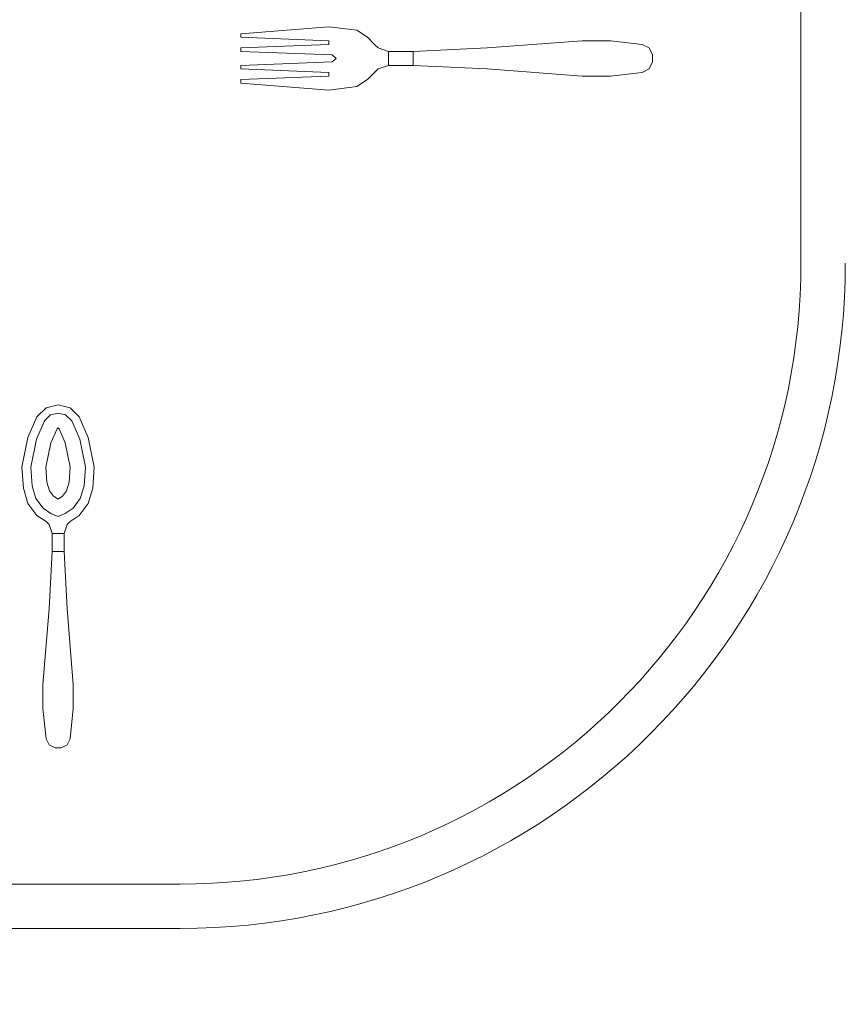
# Model space of a CAD drawing. Units: inches. Extents: x 375 to 1122, y 27 to 1069.
# Tile 17 of 155: x 732.58 to 747.02, y 253.38 to 270.59. Entities that reach past the tile are written whole.
import ezdxf

# ---------------------------------------------------------------- set-up
doc = ezdxf.new("R2010")
doc.units = ezdxf.units.IN
doc.layers.add('A-ANNO-DIMS', color=2, linetype='Continuous', lineweight=18)
doc.layers.add('Furniture', color=30, linetype='Continuous', lineweight=18)
doc.styles.get("Standard").update_dxf_attribs({"font": 'arial.ttf'})
doc.dimstyles.new('ISO-25', dxfattribs={"dimtxt": 12, "dimasz": 2.5, "dimexe": 1.5, "dimexo": 1.5, "dimtad": 1, "dimdec": 1, "dimlunit": 3, "dimtxsty": 'Standard', "dimblk": 'ARCHTICK', "dimcen": 2.5, "dimadec": 0, "dimazin": 0, "dimtfac": 1, "dimtdec": 1, "dimtmove": 0, "dimatfit": 3, "dimfxl": 1.5, "dimfxlon": 1, "dimarcsym": 0})

# ---------------------------------------------------------------- blocks, each defined once
blk = doc.blocks.new('A$C403C54AD')
for p, q in [((0.83575, 1.53256, -0.0006), (1.99923, 1.53256, -0.0006)), ((1.92199, 1.33837, -0.03581), (1.91891, 1.34298, -0.03534)), ((1.92199, 1.33837, -0.03888), (1.91891, 1.34298, -0.03842)), ((2.27071, 1.26108, -0.0006), (2.27071, 0.79569, -0.0006)), ((2.2901, 1.26108, -0.0006), (2.2901, 0.79569, -0.0006))]:
    blk.add_line(p, q)
for radius in [0.29087, 0.27148]:
    blk.add_arc((1.99923, 1.26108, -0.0006), radius, 0, 90)
for points, invisible_edges in [([(1.90506, 1.46612, -0.03397), (1.91429, 1.46612, -0.03397), (1.91583, 1.46304, -0.03421), (1.90352, 1.46304, -0.03421)], 5), ([(1.90506, 1.46612, -0.0386), (1.91429, 1.46612, -0.0386), (1.91583, 1.46304, -0.03884), (1.90352, 1.46304, -0.03884)], 5), ([(1.91121, 1.46766, -0.03413), (1.90814, 1.46766, -0.03413), (1.90506, 1.46612, -0.03397), (1.91429, 1.46612, -0.03397)], 4), ([(1.91121, 1.46766, -0.03827), (1.90814, 1.46766, -0.03827), (1.90506, 1.46612, -0.0386), (1.91429, 1.46612, -0.0386)], 4), ([(1.91583, 1.46304, -0.03421), (1.90352, 1.46304, -0.03421), (1.90198, 1.44919, -0.03425), (1.91737, 1.44919, -0.03425)], 5), ([(1.91583, 1.46304, -0.03884), (1.90352, 1.46304, -0.03884), (1.90198, 1.44919, -0.03888), (1.91737, 1.44919, -0.03888)], 5), ([(1.90198, 1.44919, -0.03425), (1.91737, 1.44919, -0.03425), (1.91737, 1.43687, -0.03392), (1.90198, 1.43687, -0.03392)], 5), ([(1.90198, 1.44919, -0.03888), (1.91737, 1.44919, -0.03888), (1.91737, 1.43687, -0.03855), (1.90198, 1.43687, -0.03855)], 5), ([(1.91737, 1.43687, -0.03392), (1.90198, 1.43687, -0.03392), (1.90506, 1.39532, -0.03153), (1.91429, 1.39532, -0.03153)], 5), ([(1.91737, 1.43687, -0.03855), (1.90198, 1.43687, -0.03855), (1.90506, 1.39532, -0.03461), (1.91429, 1.39532, -0.03461)], 5), ([(1.90198, 1.43687, -0.03855), (1.90198, 1.43687, -0.03392), (1.90506, 1.39532, -0.03153), (1.90506, 1.39532, -0.03461)], 4), ([(1.91429, 1.39532, -0.03461), (1.91429, 1.39532, -0.03153), (1.91737, 1.43687, -0.03392), (1.91737, 1.43687, -0.03855)], 1), ([(1.90506, 1.39532, -0.03153), (1.91429, 1.39532, -0.03153), (1.91275, 1.36299, -0.02863), (1.9066, 1.36299, -0.02863)], 1), ([(1.90506, 1.39532, -0.03153), (1.90506, 1.39532, -0.03461), (1.9066, 1.36299, -0.03122), (1.9066, 1.36299, -0.02863)], 5), ([(1.90506, 1.39532, -0.03461), (1.91429, 1.39532, -0.03461), (1.91275, 1.36299, -0.03122), (1.9066, 1.36299, -0.03122)], 1), ([(1.91275, 1.36299, -0.02863), (1.91275, 1.36299, -0.03122), (1.91429, 1.39532, -0.03461), (1.91429, 1.39532, -0.03153)], 5), ([(1.9066, 1.36299, -0.03122), (1.9066, 1.36299, -0.02863), (1.9066, 1.35222, -0.03071), (1.9066, 1.35222, -0.0333)], 5), ([(1.91275, 1.35222, -0.0333), (1.91275, 1.35222, -0.03071), (1.91275, 1.36299, -0.02863), (1.91275, 1.36299, -0.03122)], 5), ([(1.9066, 1.35222, -0.03071), (1.91275, 1.35222, -0.03071), (1.91429, 1.3476, -0.03306), (1.90506, 1.3476, -0.03306)], 4), ([(1.9066, 1.35222, -0.0333), (1.91275, 1.35222, -0.0333), (1.91429, 1.3476, -0.03584), (1.90506, 1.3476, -0.03584)], 4), ([(1.9066, 1.35222, -0.03071), (1.9066, 1.35222, -0.0333), (1.90506, 1.3476, -0.03584), (1.90506, 1.3476, -0.03306)], 5), ([(1.91275, 1.35222, -0.0333), (1.91275, 1.35222, -0.03071), (1.91429, 1.3476, -0.03306), (1.91429, 1.3476, -0.03584)], 5), ([(1.91429, 1.3476, -0.03306), (1.90506, 1.3476, -0.03306), (1.90352, 1.34606, -0.0341), (1.91583, 1.34606, -0.0341)], 5), ([(1.91429, 1.3476, -0.03584), (1.90506, 1.3476, -0.03584), (1.90352, 1.34606, -0.03718), (1.91583, 1.34606, -0.03718)], 5), ([(1.90506, 1.3476, -0.03584), (1.90506, 1.3476, -0.03306), (1.90352, 1.34606, -0.0341), (1.90352, 1.34606, -0.03718)], 1), ([(1.91429, 1.3476, -0.03306), (1.91429, 1.3476, -0.03584), (1.91583, 1.34606, -0.03718), (1.91583, 1.34606, -0.0341)], 1), ([(1.91583, 1.34606, -0.03718), (1.90352, 1.34606, -0.03718), (1.90044, 1.34298, -0.03842), (1.91891, 1.34298, -0.03842)], 5), ([(1.91583, 1.34606, -0.0341), (1.90352, 1.34606, -0.0341), (1.90044, 1.34298, -0.03534), (1.91891, 1.34298, -0.03534)], 5), ([(1.90044, 1.34298, -0.03534), (1.91891, 1.34298, -0.03534), (1.92199, 1.33837, -0.03581), (1.89736, 1.33837, -0.03581)], 5), ([(1.90044, 1.34298, -0.03842), (1.91891, 1.34298, -0.03842), (1.92199, 1.33837, -0.03888), (1.89736, 1.33837, -0.03888)], 5), ([(1.90044, 1.34298, -0.03842), (1.90044, 1.34298, -0.03534), (1.89736, 1.33837, -0.03581), (1.89736, 1.33837, -0.03888)], 4), ([(1.91891, 1.34298, -0.03534), (1.91891, 1.34298, -0.03842), (1.92199, 1.33837, -0.03888), (1.92199, 1.33837, -0.03581)], 4), ([(1.89736, 1.33837, -0.03581), (1.90352, 1.32605, -0.03521), (1.90198, 1.32605, -0.03521), (1.89582, 1.32605, -0.03521)], 5), ([(1.89736, 1.33837, -0.03888), (1.90352, 1.32605, -0.03829), (1.90198, 1.32605, -0.03829), (1.89582, 1.32605, -0.03829)], 5), ([(1.89736, 1.33837, -0.03581), (1.89736, 1.33837, -0.03888), (1.89582, 1.32605, -0.03829), (1.89582, 1.32605, -0.03521)], 1), ([(1.89736, 1.33837, -0.03581), (1.90968, 1.32925, -0.0356), (1.90814, 1.32759, -0.03545), (1.90352, 1.32605, -0.03521)], 13), ([(1.89736, 1.33837, -0.03581), (1.90968, 1.32925, -0.0356), (1.92199, 1.33837, -0.03581), (1.89736, 1.33837, -0.03581)], 7), ([(1.89736, 1.33837, -0.03888), (1.90968, 1.32925, -0.03868), (1.90814, 1.32759, -0.03853), (1.90352, 1.32605, -0.03829)], 13), ([(1.89736, 1.33837, -0.03888), (1.90968, 1.32925, -0.03868), (1.92199, 1.33837, -0.03888), (1.89736, 1.33837, -0.03888)], 7), ([(1.92199, 1.33837, -0.03581), (1.90968, 1.32925, -0.0356), (1.91121, 1.32759, -0.03545), (1.91583, 1.32605, -0.03521)], 13), ([(1.92199, 1.33837, -0.03888), (1.90968, 1.32925, -0.03868), (1.91121, 1.32759, -0.03853), (1.91583, 1.32605, -0.03829)], 13), ([(1.92199, 1.33837, -0.03581), (1.91583, 1.32605, -0.03521), (1.91737, 1.32605, -0.03521), (1.92353, 1.32605, -0.03521)], 5), ([(1.92199, 1.33837, -0.03888), (1.91583, 1.32605, -0.03829), (1.91737, 1.32605, -0.03829), (1.92353, 1.32605, -0.03829)], 5), ([(1.92199, 1.33837, -0.03888), (1.92199, 1.33837, -0.03581), (1.92353, 1.32605, -0.03521), (1.92353, 1.32605, -0.03829)], 1), ([(1.90198, 1.32605, -0.03521), (1.89582, 1.32605, -0.03521), (1.8989, 1.28757, -0.02811), (1.90044, 1.28757, -0.02811)], 1), ([(1.90198, 1.32605, -0.03829), (1.89582, 1.32605, -0.03829), (1.8989, 1.28757, -0.03119), (1.90044, 1.28757, -0.03119)], 1), ([(1.90352, 1.32605, -0.03521), (1.90814, 1.32759, -0.03545), (1.9066, 1.28757, -0.02811), (1.90506, 1.28757, -0.02811)], 1), ([(1.90352, 1.32605, -0.03829), (1.90814, 1.32759, -0.03853), (1.9066, 1.28757, -0.03119), (1.90506, 1.28757, -0.03119)], 1), ([(1.91121, 1.32759, -0.03545), (1.91583, 1.32605, -0.03521), (1.91429, 1.28757, -0.02811), (1.91275, 1.28757, -0.02811)], 1), ([(1.91121, 1.32759, -0.03853), (1.91583, 1.32605, -0.03829), (1.91429, 1.28757, -0.03119), (1.91275, 1.28757, -0.03119)], 1), ([(1.91737, 1.32605, -0.03521), (1.92353, 1.32605, -0.03521), (1.92045, 1.28757, -0.02811), (1.91891, 1.28757, -0.02811)], 1), ([(1.91737, 1.32605, -0.03829), (1.92353, 1.32605, -0.03829), (1.92045, 1.28757, -0.03119), (1.91891, 1.28757, -0.03119)], 1), ([(2.08833, 1.21962, -0.05699), (2.08844, 1.2235, -0.05453), (2.0754, 1.22086, -0.05249), (2.0762, 1.21716, -0.05501)], 5), ([(2.08833, 1.21962, -0.05567), (2.08844, 1.2235, -0.05321), (2.0754, 1.22086, -0.05117), (2.0762, 1.21716, -0.05369)], 5), ([(2.09764, 1.22284, -0.05408), (2.09658, 1.21902, -0.05656), (2.08833, 1.21962, -0.05567), (2.08844, 1.2235, -0.05321)], 5), ([(2.09764, 1.22284, -0.0554), (2.09658, 1.21902, -0.05788), (2.08833, 1.21962, -0.05699), (2.08844, 1.2235, -0.05453)], 5), ([(2.1021, 1.21736, -0.05707), (2.10425, 1.22086, -0.05448), (2.09764, 1.22284, -0.05408), (2.09658, 1.21902, -0.05656)], 5), ([(2.1021, 1.21736, -0.05839), (2.10425, 1.22086, -0.0558), (2.09764, 1.22284, -0.0554), (2.09658, 1.21902, -0.05788)], 5), ([(2.0754, 1.22086, -0.05249), (2.0762, 1.21716, -0.05501), (2.06818, 1.21365, -0.0533), (2.06633, 1.2169, -0.05066)], 5), ([(2.0754, 1.22086, -0.05117), (2.0762, 1.21716, -0.05369), (2.06818, 1.21365, -0.05198), (2.06633, 1.2169, -0.04934)], 5), ([(2.07778, 1.21084, -0.0565), (2.0762, 1.21716, -0.05369), (2.08833, 1.21962, -0.05567), (2.08839, 1.21299, -0.05821)], 5), ([(2.07778, 1.21084, -0.05782), (2.0762, 1.21716, -0.05501), (2.08833, 1.21962, -0.05699), (2.08839, 1.21299, -0.05953)], 5), ([(2.08833, 1.21962, -0.05699), (2.08839, 1.21299, -0.05953), (2.095, 1.21251, -0.06048), (2.09658, 1.21902, -0.05788)], 5), ([(2.08833, 1.21962, -0.05567), (2.08839, 1.21299, -0.05821), (2.095, 1.21251, -0.05916), (2.09658, 1.21902, -0.05656)], 5), ([(2.095, 1.21251, -0.06048), (2.09658, 1.21902, -0.05788), (2.1021, 1.21736, -0.05839), (2.09872, 1.2114, -0.06071)], 5), ([(2.095, 1.21251, -0.05916), (2.09658, 1.21902, -0.05656), (2.1021, 1.21736, -0.05707), (2.09872, 1.2114, -0.05939)], 5), ([(2.10951, 1.2169, -0.05628), (2.10632, 1.21421, -0.05856), (2.1021, 1.21736, -0.05839), (2.10425, 1.22086, -0.0558)], 5), ([(2.10951, 1.2169, -0.05496), (2.10632, 1.21421, -0.05724), (2.1021, 1.21736, -0.05707), (2.10425, 1.22086, -0.05448)], 5), ([(2.06818, 1.21365, -0.0533), (2.06633, 1.2169, -0.05066), (2.06249, 1.21294, -0.04957), (2.06555, 1.21097, -0.05274)], 5), ([(2.06818, 1.21365, -0.05198), (2.06633, 1.2169, -0.04934), (2.06249, 1.21294, -0.04825), (2.06555, 1.21097, -0.05142)], 5), ([(2.06818, 1.21365, -0.0533), (2.07156, 1.2081, -0.05619), (2.07778, 1.21084, -0.05782), (2.0762, 1.21716, -0.05501)], 5), ([(2.06818, 1.21365, -0.05198), (2.07156, 1.2081, -0.05487), (2.07778, 1.21084, -0.0565), (2.0762, 1.21716, -0.05369)], 5), ([(2.1021, 1.21736, -0.05839), (2.09872, 1.2114, -0.06071), (2.1011, 1.20963, -0.06081), (2.10632, 1.21421, -0.05856)], 5), ([(2.1021, 1.21736, -0.05707), (2.09872, 1.2114, -0.05939), (2.1011, 1.20963, -0.05949), (2.10632, 1.21421, -0.05724)], 5), ([(2.1011, 1.20963, -0.06081), (2.10632, 1.21421, -0.05856), (2.10861, 1.2108, -0.05857), (2.10244, 1.20767, -0.06061)], 5), ([(2.1011, 1.20963, -0.05949), (2.10632, 1.21421, -0.05724), (2.10861, 1.2108, -0.05725), (2.10244, 1.20767, -0.05929)], 5), ([(2.10861, 1.2108, -0.05857), (2.11212, 1.21294, -0.05749), (2.10951, 1.2169, -0.05628), (2.10632, 1.21421, -0.05856)], 5), ([(2.10861, 1.2108, -0.05725), (2.11212, 1.21294, -0.05534), (2.10951, 1.2169, -0.05496), (2.10632, 1.21421, -0.05724)], 5), ([(2.18338, 1.20107, -0.06063), (2.18338, 1.21426, -0.06063), (2.1504, 1.21162, -0.05725), (2.1504, 1.20371, -0.05725)], 5), ([(2.18338, 1.21426, -0.06063), (2.18338, 1.21426, -0.05666), (2.1504, 1.21162, -0.05462), (2.1504, 1.21162, -0.05725)], 4), ([(2.18338, 1.20107, -0.05666), (2.18338, 1.21426, -0.05666), (2.1504, 1.21162, -0.05462), (2.1504, 1.20371, -0.05462)], 5), ([(2.19393, 1.21426, -0.05694), (2.19393, 1.20107, -0.05694), (2.18338, 1.20107, -0.05666), (2.18338, 1.21426, -0.05666)], 5), ([(2.19393, 1.21426, -0.06091), (2.19393, 1.20107, -0.06091), (2.18338, 1.20107, -0.06063), (2.18338, 1.21426, -0.06063)], 5), ([(2.20713, 1.20239, -0.05691), (2.20713, 1.21294, -0.05691), (2.19393, 1.21426, -0.05694), (2.19393, 1.20107, -0.05694)], 5), ([(2.20713, 1.20239, -0.06088), (2.20713, 1.21294, -0.06088), (2.19393, 1.21426, -0.06091), (2.19393, 1.20107, -0.06091)], 5), ([(2.06249, 1.21294, -0.04957), (2.06555, 1.21097, -0.05274), (2.06475, 1.20767, -0.05255), (2.06119, 1.20767, -0.04938)], 5), ([(2.06249, 1.21294, -0.04825), (2.06555, 1.21097, -0.05142), (2.06475, 1.20767, -0.05124), (2.06119, 1.20767, -0.04806)], 5), ([(2.06475, 1.20767, -0.05124), (2.07114, 1.20767, -0.05473), (2.07156, 1.2081, -0.05487), (2.06555, 1.21097, -0.05142)], 5), ([(2.06475, 1.20767, -0.05255), (2.07114, 1.20767, -0.05605), (2.07156, 1.2081, -0.05619), (2.06555, 1.21097, -0.05274)], 5), ([(2.07156, 1.2081, -0.05487), (2.06555, 1.21097, -0.05142), (2.06818, 1.21365, -0.05198), (2.07156, 1.2081, -0.05487)], 5), ([(2.07156, 1.2081, -0.05619), (2.06555, 1.21097, -0.05274), (2.06818, 1.21365, -0.0533), (2.07156, 1.2081, -0.05619)], 5), ([(2.07156, 1.20723, -0.05619), (2.07156, 1.2081, -0.05619), (2.07778, 1.21084, -0.05782), (2.07778, 1.20449, -0.05782)], 5), ([(2.07156, 1.20723, -0.05487), (2.07156, 1.2081, -0.05487), (2.07778, 1.21084, -0.0565), (2.07778, 1.20449, -0.0565)], 5), ([(2.07778, 1.21084, -0.0565), (2.07778, 1.20449, -0.0565), (2.08839, 1.20234, -0.05821), (2.08839, 1.21299, -0.05821)], 5), ([(2.07778, 1.21084, -0.05782), (2.07778, 1.20449, -0.05782), (2.08839, 1.20234, -0.05953), (2.08839, 1.21299, -0.05953)], 5), ([(2.08839, 1.20234, -0.05953), (2.08839, 1.21299, -0.05953), (2.095, 1.21251, -0.06048), (2.095, 1.20282, -0.06048)], 5), ([(2.08839, 1.20234, -0.05821), (2.08839, 1.21299, -0.05821), (2.095, 1.21251, -0.05916), (2.095, 1.20282, -0.05916)], 5), ([(2.095, 1.21251, -0.06048), (2.095, 1.20282, -0.06048), (2.09872, 1.20393, -0.06071), (2.09872, 1.2114, -0.06071)], 5), ([(2.095, 1.21251, -0.05916), (2.095, 1.20282, -0.05916), (2.09872, 1.20393, -0.05939), (2.09872, 1.2114, -0.05939)], 5), ([(2.09872, 1.20393, -0.06071), (2.09872, 1.2114, -0.06071), (2.1011, 1.20963, -0.06081), (2.1011, 1.2057, -0.06081)], 5), ([(2.09872, 1.20393, -0.05939), (2.09872, 1.2114, -0.05939), (2.1011, 1.20963, -0.05949), (2.1011, 1.2057, -0.05949)], 5), ([(2.10861, 1.2108, -0.05857), (2.10244, 1.20767, -0.06061), (2.10244, 1.20767, -0.06061), (2.10997, 1.20767, -0.05839)], 5), ([(2.10861, 1.2108, -0.05725), (2.10244, 1.20767, -0.05929), (2.10244, 1.20767, -0.05929), (2.10997, 1.20767, -0.05707)], 5), ([(2.11212, 1.21294, -0.05749), (2.11212, 1.20767, -0.05749), (2.10997, 1.20767, -0.05839), (2.10861, 1.2108, -0.05857)], 11), ([(2.11212, 1.21294, -0.05534), (2.11212, 1.20767, -0.05534), (2.10997, 1.20767, -0.05707), (2.10861, 1.2108, -0.05725)], 11), ([(2.11345, 1.20371, -0.0546), (2.11345, 1.21162, -0.0546), (2.11212, 1.21294, -0.05534), (2.11212, 1.20239, -0.05534)], 5), ([(2.11345, 1.20371, -0.05669), (2.11345, 1.21162, -0.05669), (2.11212, 1.21294, -0.05749), (2.11212, 1.20239, -0.05749)], 5), ([(2.11345, 1.21162, -0.05669), (2.11345, 1.21162, -0.0546), (2.11212, 1.21294, -0.05534), (2.11212, 1.21294, -0.05749)], 1), ([(2.11741, 1.2103, -0.05275), (2.11741, 1.20503, -0.05275), (2.11345, 1.20371, -0.0546), (2.11345, 1.21162, -0.0546)], 4), ([(2.11741, 1.2103, -0.05275), (2.11741, 1.2103, -0.05497), (2.11345, 1.21162, -0.05669), (2.11345, 1.21162, -0.0546)], 5), ([(2.11741, 1.2103, -0.05497), (2.11741, 1.20503, -0.05497), (2.11345, 1.20371, -0.05669), (2.11345, 1.21162, -0.05669)], 4), ([(2.12533, 1.2103, -0.05434), (2.12533, 1.2103, -0.05212), (2.11741, 1.2103, -0.05275), (2.11741, 1.2103, -0.05497)], 5), ([(2.1504, 1.21162, -0.05462), (2.1504, 1.20371, -0.05462), (2.12533, 1.20503, -0.05212), (2.12533, 1.2103, -0.05212)], 1), ([(2.1504, 1.21162, -0.05462), (2.1504, 1.21162, -0.05725), (2.12533, 1.2103, -0.05434), (2.12533, 1.2103, -0.05212)], 5), ([(2.1504, 1.21162, -0.05725), (2.1504, 1.20371, -0.05725), (2.12533, 1.20503, -0.05434), (2.12533, 1.2103, -0.05434)], 1), ([(2.20976, 1.21162, -0.0567), (2.20976, 1.20371, -0.0567), (2.20713, 1.20239, -0.05691), (2.20713, 1.21294, -0.05691)], 5), ([(2.20976, 1.21162, -0.06067), (2.20976, 1.20371, -0.06067), (2.20713, 1.20239, -0.06088), (2.20713, 1.21294, -0.06088)], 5), ([(2.21108, 1.20635, -0.05684), (2.21108, 1.20898, -0.05684), (2.20976, 1.21162, -0.0567), (2.20976, 1.20371, -0.0567)], 4), ([(2.21108, 1.20635, -0.06038), (2.21108, 1.20898, -0.06038), (2.20976, 1.21162, -0.06067), (2.20976, 1.20371, -0.06067)], 4), ([(2.06249, 1.20239, -0.04957), (2.06555, 1.20436, -0.05274), (2.06475, 1.20767, -0.05255), (2.06119, 1.20767, -0.04938)], 5), ([(2.06249, 1.20239, -0.04825), (2.06555, 1.20436, -0.05142), (2.06475, 1.20767, -0.05124), (2.06119, 1.20767, -0.04806)], 5), ([(2.06475, 1.20767, -0.05124), (2.07114, 1.20767, -0.05473), (2.07156, 1.20723, -0.05487), (2.06555, 1.20436, -0.05142)], 5), ([(2.06475, 1.20767, -0.05255), (2.07114, 1.20767, -0.05605), (2.07156, 1.20723, -0.05619), (2.06555, 1.20436, -0.05274)], 5), ([(2.07156, 1.20723, -0.05487), (2.06555, 1.20436, -0.05142), (2.06818, 1.20168, -0.05198), (2.07156, 1.20723, -0.05487)], 5), ([(2.07156, 1.20723, -0.05619), (2.06555, 1.20436, -0.05274), (2.06818, 1.20168, -0.0533), (2.07156, 1.20723, -0.05619)], 5), ([(2.06818, 1.20168, -0.0533), (2.07156, 1.20723, -0.05619), (2.07778, 1.20449, -0.05782), (2.0762, 1.19817, -0.05501)], 5), ([(2.06818, 1.20168, -0.05198), (2.07156, 1.20723, -0.05487), (2.07778, 1.20449, -0.0565), (2.0762, 1.19817, -0.05369)], 5), ([(2.07114, 1.20767, -0.05473), (2.07156, 1.2081, -0.05487), (2.07156, 1.20723, -0.05487), (2.07114, 1.20767, -0.05473)], 2), ([(2.07114, 1.20767, -0.05605), (2.07156, 1.2081, -0.05619), (2.07156, 1.20723, -0.05619), (2.07114, 1.20767, -0.05605)], 2), ([(2.1021, 1.19797, -0.05839), (2.09872, 1.20393, -0.06071), (2.1011, 1.2057, -0.06081), (2.10632, 1.20112, -0.05856)], 5), ([(2.1021, 1.19797, -0.05707), (2.09872, 1.20393, -0.05939), (2.1011, 1.2057, -0.05949), (2.10632, 1.20112, -0.05724)], 5), ([(2.1011, 1.20963, -0.06081), (2.1011, 1.2057, -0.06081), (2.10244, 1.20767, -0.06061)], 1), ([(2.1011, 1.20963, -0.05949), (2.1011, 1.2057, -0.05949), (2.10244, 1.20767, -0.05929)], 1), ([(2.1011, 1.2057, -0.06081), (2.10632, 1.20112, -0.05856), (2.10861, 1.20453, -0.05857), (2.10244, 1.20767, -0.06061)], 5), ([(2.1011, 1.2057, -0.05949), (2.10632, 1.20112, -0.05724), (2.10861, 1.20453, -0.05725), (2.10244, 1.20767, -0.05929)], 5), ([(2.10861, 1.20453, -0.05857), (2.10244, 1.20767, -0.06061), (2.10244, 1.20767, -0.06061), (2.10997, 1.20767, -0.05839)], 5), ([(2.10861, 1.20453, -0.05725), (2.10244, 1.20767, -0.05929), (2.10244, 1.20767, -0.05929), (2.10997, 1.20767, -0.05707)], 5), ([(2.11212, 1.20239, -0.05749), (2.11212, 1.20767, -0.05749), (2.10997, 1.20767, -0.05839), (2.10861, 1.20453, -0.05857)], 11), ([(2.11212, 1.20239, -0.05534), (2.11212, 1.20767, -0.05534), (2.10997, 1.20767, -0.05707), (2.10861, 1.20453, -0.05725)], 11), ([(2.06818, 1.20168, -0.0533), (2.06633, 1.19843, -0.05066), (2.06249, 1.20239, -0.04957), (2.06555, 1.20436, -0.05274)], 5), ([(2.06818, 1.20168, -0.05198), (2.06633, 1.19843, -0.04934), (2.06249, 1.20239, -0.04825), (2.06555, 1.20436, -0.05142)], 5), ([(2.0754, 1.19447, -0.05249), (2.0762, 1.19817, -0.05501), (2.06818, 1.20168, -0.0533), (2.06633, 1.19843, -0.05066)], 5), ([(2.0754, 1.19447, -0.05117), (2.0762, 1.19817, -0.05369), (2.06818, 1.20168, -0.05198), (2.06633, 1.19843, -0.04934)], 5), ([(2.07778, 1.20449, -0.0565), (2.0762, 1.19817, -0.05369), (2.08833, 1.19571, -0.05567), (2.08839, 1.20234, -0.05821)], 5), ([(2.07778, 1.20449, -0.05782), (2.0762, 1.19817, -0.05501), (2.08833, 1.19571, -0.05699), (2.08839, 1.20234, -0.05953)], 5), ([(2.08833, 1.19571, -0.05699), (2.08839, 1.20234, -0.05953), (2.095, 1.20282, -0.06048), (2.09658, 1.19631, -0.05788)], 5), ([(2.08833, 1.19571, -0.05567), (2.08839, 1.20234, -0.05821), (2.095, 1.20282, -0.05916), (2.09658, 1.19631, -0.05656)], 5), ([(2.095, 1.20282, -0.05916), (2.09658, 1.19631, -0.05656), (2.1021, 1.19797, -0.05707), (2.09872, 1.20393, -0.05939)], 5), ([(2.10861, 1.20453, -0.05725), (2.11212, 1.20239, -0.05534), (2.10951, 1.19843, -0.05496), (2.10632, 1.20112, -0.05724)], 5), ([(2.11345, 1.20371, -0.0546), (2.11345, 1.20371, -0.05669), (2.11212, 1.20239, -0.05749), (2.11212, 1.20239, -0.05534)], 1), ([(2.11741, 1.20503, -0.05497), (2.11741, 1.20503, -0.05275), (2.11345, 1.20371, -0.0546), (2.11345, 1.20371, -0.05669)], 5), ([(2.11741, 1.20503, -0.05497), (2.11741, 1.20503, -0.05275), (2.12533, 1.20503, -0.05212), (2.12533, 1.20503, -0.05434)], 5), ([(2.12533, 1.20503, -0.05212), (2.12533, 1.20503, -0.05434), (2.1504, 1.20371, -0.05725), (2.1504, 1.20371, -0.05462)], 5), ([(2.1504, 1.20371, -0.05725), (2.1504, 1.20371, -0.05462), (2.18338, 1.20107, -0.05666), (2.18338, 1.20107, -0.06063)], 1), ([(2.08833, 1.19571, -0.05699), (2.08844, 1.19183, -0.05453), (2.0754, 1.19447, -0.05249), (2.0762, 1.19817, -0.05501)], 5), ([(2.08833, 1.19571, -0.05567), (2.08844, 1.19183, -0.05321), (2.0754, 1.19447, -0.05117), (2.0762, 1.19817, -0.05369)], 5), ([(2.1021, 1.19797, -0.05707), (2.10425, 1.19447, -0.05448), (2.09764, 1.19249, -0.05408), (2.09658, 1.19631, -0.05656)], 5), ([(2.1021, 1.19797, -0.05839), (2.10425, 1.19447, -0.0558), (2.09764, 1.19249, -0.0554), (2.09658, 1.19631, -0.05788)], 5), ([(2.10951, 1.19843, -0.05628), (2.10632, 1.20112, -0.05856), (2.1021, 1.19797, -0.05839), (2.10425, 1.19447, -0.0558)], 5), ([(2.10951, 1.19843, -0.05496), (2.10632, 1.20112, -0.05724), (2.1021, 1.19797, -0.05707), (2.10425, 1.19447, -0.05448)], 5), ([(2.09764, 1.19249, -0.05408), (2.09658, 1.19631, -0.05656), (2.08833, 1.19571, -0.05567), (2.08844, 1.19183, -0.05321)], 5), ([(2.09764, 1.19249, -0.0554), (2.09658, 1.19631, -0.05788), (2.08833, 1.19571, -0.05699), (2.08844, 1.19183, -0.05453)], 5)]:
    blk.add_3dface(points, dxfattribs=dict(invisible_edges=invisible_edges))
for points in [[(1.90506, 1.46612, -0.03397), (1.90506, 1.46612, -0.0386), (1.90352, 1.46304, -0.03884), (1.90352, 1.46304, -0.03421)], [(1.90814, 1.46766, -0.03827), (1.90814, 1.46766, -0.03413), (1.90506, 1.46612, -0.03397), (1.90506, 1.46612, -0.0386)], [(1.91121, 1.46766, -0.03413), (1.91121, 1.46766, -0.03827), (1.90814, 1.46766, -0.03827), (1.90814, 1.46766, -0.03413)], [(1.91429, 1.46612, -0.0386), (1.91429, 1.46612, -0.03397), (1.91121, 1.46766, -0.03413), (1.91121, 1.46766, -0.03827)], [(1.91583, 1.46304, -0.03421), (1.91583, 1.46304, -0.03884), (1.91429, 1.46612, -0.0386), (1.91429, 1.46612, -0.03397)], [(1.90352, 1.46304, -0.03884), (1.90352, 1.46304, -0.03421), (1.90198, 1.44919, -0.03425), (1.90198, 1.44919, -0.03888)], [(1.91737, 1.44919, -0.03888), (1.91737, 1.44919, -0.03425), (1.91583, 1.46304, -0.03421), (1.91583, 1.46304, -0.03884)], [(1.90198, 1.44919, -0.03425), (1.90198, 1.44919, -0.03888), (1.90198, 1.43687, -0.03855), (1.90198, 1.43687, -0.03392)], [(1.91737, 1.43687, -0.03392), (1.91737, 1.43687, -0.03855), (1.91737, 1.44919, -0.03888), (1.91737, 1.44919, -0.03425)], [(1.91275, 1.36299, -0.02863), (1.9066, 1.36299, -0.02863), (1.9066, 1.35222, -0.03071), (1.91275, 1.35222, -0.03071)], [(1.91275, 1.36299, -0.03122), (1.9066, 1.36299, -0.03122), (1.9066, 1.35222, -0.0333), (1.91275, 1.35222, -0.0333)], [(1.90352, 1.34606, -0.0341), (1.90352, 1.34606, -0.03718), (1.90044, 1.34298, -0.03842), (1.90044, 1.34298, -0.03534)], [(1.91583, 1.34606, -0.03718), (1.91583, 1.34606, -0.0341), (1.91891, 1.34298, -0.03534), (1.91891, 1.34298, -0.03842)], [(1.89582, 1.32605, -0.03829), (1.89582, 1.32605, -0.03521), (1.8989, 1.28757, -0.02811), (1.8989, 1.28757, -0.03119)], [(1.90044, 1.28757, -0.02811), (1.90044, 1.28757, -0.03119), (1.90198, 1.32605, -0.03829), (1.90198, 1.32605, -0.03521)], [(1.90352, 1.32605, -0.03829), (1.90352, 1.32605, -0.03521), (1.90198, 1.32605, -0.03521), (1.90198, 1.32605, -0.03829)], [(1.90352, 1.32605, -0.03829), (1.90352, 1.32605, -0.03521), (1.90506, 1.28757, -0.02811), (1.90506, 1.28757, -0.03119)], [(1.9066, 1.28757, -0.03119), (1.9066, 1.28757, -0.02811), (1.90814, 1.32759, -0.03545), (1.90814, 1.32759, -0.03853)], [(1.90968, 1.32925, -0.03868), (1.90968, 1.32925, -0.0356), (1.90814, 1.32759, -0.03545), (1.90814, 1.32759, -0.03853)], [(1.91121, 1.32759, -0.03545), (1.91121, 1.32759, -0.03853), (1.90968, 1.32925, -0.03868), (1.90968, 1.32925, -0.0356)], [(1.91121, 1.32759, -0.03853), (1.91121, 1.32759, -0.03545), (1.91275, 1.28757, -0.02811), (1.91275, 1.28757, -0.03119)], [(1.91429, 1.28757, -0.02811), (1.91429, 1.28757, -0.03119), (1.91583, 1.32605, -0.03829), (1.91583, 1.32605, -0.03521)], [(1.91737, 1.32605, -0.03521), (1.91737, 1.32605, -0.03829), (1.91583, 1.32605, -0.03829), (1.91583, 1.32605, -0.03521)], [(1.91737, 1.32605, -0.03521), (1.91737, 1.32605, -0.03829), (1.91891, 1.28757, -0.03119), (1.91891, 1.28757, -0.02811)], [(1.92045, 1.28757, -0.02811), (1.92045, 1.28757, -0.03119), (1.92353, 1.32605, -0.03829), (1.92353, 1.32605, -0.03521)], [(1.8989, 1.28757, -0.03119), (1.8989, 1.28757, -0.02811), (1.90044, 1.28757, -0.02811), (1.90044, 1.28757, -0.03119)], [(1.90506, 1.28757, -0.03119), (1.90506, 1.28757, -0.02811), (1.9066, 1.28757, -0.02811), (1.9066, 1.28757, -0.03119)], [(1.91275, 1.28757, -0.03119), (1.91275, 1.28757, -0.02811), (1.91429, 1.28757, -0.02811), (1.91429, 1.28757, -0.03119)], [(1.91891, 1.28757, -0.03119), (1.91891, 1.28757, -0.02811), (1.92045, 1.28757, -0.02811), (1.92045, 1.28757, -0.03119)], [(2.08844, 1.2235, -0.05453), (2.08844, 1.2235, -0.05321), (2.0754, 1.22086, -0.05117), (2.0754, 1.22086, -0.05249)], [(2.09764, 1.22284, -0.05408), (2.09764, 1.22284, -0.0554), (2.08844, 1.2235, -0.05453), (2.08844, 1.2235, -0.05321)], [(2.10425, 1.22086, -0.0558), (2.10425, 1.22086, -0.05448), (2.09764, 1.22284, -0.05408), (2.09764, 1.22284, -0.0554)], [(2.0754, 1.22086, -0.05117), (2.0754, 1.22086, -0.05249), (2.06633, 1.2169, -0.05066), (2.06633, 1.2169, -0.04934)], [(2.10951, 1.2169, -0.05496), (2.10951, 1.2169, -0.05628), (2.10425, 1.22086, -0.0558), (2.10425, 1.22086, -0.05448)], [(2.06633, 1.2169, -0.05066), (2.06633, 1.2169, -0.04934), (2.06249, 1.21294, -0.04825), (2.06249, 1.21294, -0.04957)], [(2.11212, 1.21294, -0.05749), (2.11212, 1.21294, -0.05534), (2.10951, 1.2169, -0.05496), (2.10951, 1.2169, -0.05628)], [(2.19393, 1.21426, -0.05694), (2.19393, 1.21426, -0.06091), (2.18338, 1.21426, -0.06063), (2.18338, 1.21426, -0.05666)], [(2.20713, 1.21294, -0.06088), (2.20713, 1.21294, -0.05691), (2.19393, 1.21426, -0.05694), (2.19393, 1.21426, -0.06091)], [(2.06249, 1.21294, -0.04825), (2.06249, 1.21294, -0.04957), (2.06119, 1.20767, -0.04938), (2.06119, 1.20767, -0.04806)], [(2.12533, 1.20503, -0.05434), (2.12533, 1.2103, -0.05434), (2.11741, 1.2103, -0.05497), (2.11741, 1.20503, -0.05497)], [(2.12533, 1.20503, -0.05212), (2.12533, 1.2103, -0.05212), (2.11741, 1.2103, -0.05275), (2.11741, 1.20503, -0.05275)], [(2.20976, 1.21162, -0.0567), (2.20976, 1.21162, -0.06067), (2.20713, 1.21294, -0.06088), (2.20713, 1.21294, -0.05691)], [(2.21108, 1.20898, -0.06038), (2.21108, 1.20898, -0.05684), (2.20976, 1.21162, -0.0567), (2.20976, 1.21162, -0.06067)], [(2.06119, 1.20767, -0.04938), (2.06119, 1.20767, -0.04806), (2.06249, 1.20239, -0.04825), (2.06249, 1.20239, -0.04957)], [(2.20976, 1.20371, -0.06067), (2.20976, 1.20371, -0.0567), (2.21108, 1.20635, -0.05684), (2.21108, 1.20635, -0.06038)], [(2.21108, 1.20635, -0.05684), (2.21108, 1.20635, -0.06038), (2.21108, 1.20898, -0.06038), (2.21108, 1.20898, -0.05684)], [(2.06249, 1.20239, -0.04825), (2.06249, 1.20239, -0.04957), (2.06633, 1.19843, -0.05066), (2.06633, 1.19843, -0.04934)], [(2.10951, 1.19843, -0.05628), (2.10951, 1.19843, -0.05496), (2.11212, 1.20239, -0.05534), (2.11212, 1.20239, -0.05749)], [(2.19393, 1.20107, -0.06091), (2.19393, 1.20107, -0.05694), (2.20713, 1.20239, -0.05691), (2.20713, 1.20239, -0.06088)], [(2.20713, 1.20239, -0.05691), (2.20713, 1.20239, -0.06088), (2.20976, 1.20371, -0.06067), (2.20976, 1.20371, -0.0567)], [(2.06633, 1.19843, -0.05066), (2.06633, 1.19843, -0.04934), (2.0754, 1.19447, -0.05117), (2.0754, 1.19447, -0.05249)], [(2.10425, 1.19447, -0.05448), (2.10425, 1.19447, -0.0558), (2.10951, 1.19843, -0.05628), (2.10951, 1.19843, -0.05496)], [(2.18338, 1.20107, -0.05666), (2.18338, 1.20107, -0.06063), (2.19393, 1.20107, -0.06091), (2.19393, 1.20107, -0.05694)], [(2.0754, 1.19447, -0.05117), (2.0754, 1.19447, -0.05249), (2.08844, 1.19183, -0.05453), (2.08844, 1.19183, -0.05321)], [(2.09764, 1.19249, -0.0554), (2.09764, 1.19249, -0.05408), (2.10425, 1.19447, -0.05448), (2.10425, 1.19447, -0.0558)], [(2.08844, 1.19183, -0.05453), (2.08844, 1.19183, -0.05321), (2.09764, 1.19249, -0.05408), (2.09764, 1.19249, -0.0554)]]:
    blk.add_3dface(points)
blk = doc.blocks.new('_ArchTick')
at = {"color": 0, "linetype": 'ByBlock', "const_width": 0.15}
blk.add_lwpolyline([(-0.5, -0.5), (0.5, 0.5)], dxfattribs=at)
blk = doc.blocks.new('*D94')
at = {"layer": 'A-ANNO-DIMS', "color": 0, "lineweight": -2, "transparency": 16777216}
for p, q in [((734.007, 117.528), (734.007, 114.528)), ((773.007, 117.528), (773.007, 114.528)), ((734.007, 116.028), (773.007, 116.028))]:
    blk.add_line(p, q, dxfattribs=at)
at = {"layer": 'Defpoints', "color": 0, "transparency": 16777216}
for p in [(734.007, 667.528), (773.007, 667.528), (773.007, 116.028)]:
    blk.add_point(p, dxfattribs=at)
at = {"layer": 'A-ANNO-DIMS', "color": 0, "lineweight": -2, "transparency": 16777216, "xscale": 2.5, "yscale": 2.5, "zscale": 2.5, "rotation": 180}
blk.add_blockref('_ArchTick', (734.007, 116.028), dxfattribs=at)
at = {"layer": 'A-ANNO-DIMS', "color": 0, "lineweight": -2, "transparency": 16777216, "xscale": 2.5, "yscale": 2.5, "zscale": 2.5}
blk.add_blockref('_ArchTick', (773.007, 116.028), dxfattribs=at)
at = {"layer": 'A-ANNO-DIMS', "color": 0, "transparency": 16777216, "insert": (753.507, 122.784), "char_height": 12, "attachment_point": 5}
blk.add_mtext('3\'-3"', dxfattribs=at)

msp = doc.modelspace()

# ---------------------------------------------------------------- block references
at = {"layer": 'Furniture', "xscale": 39.9918517141215, "yscale": 39.9918517141215, "zscale": 39.9918517141215, "rotation": 270}
msp.add_blockref('A$C403C54AD', (684.955, 346.287, 0.024), dxfattribs=at)

# ---------------------------------------------------------------- dimensions: what is measured, and where the dimension line sits
at = {"layer": 'A-ANNO-DIMS'}
dim = msp.add_linear_dim(base=(773.007, 116.028), p1=(734.007, 667.528), p2=(773.007, 667.528), dimstyle='ISO-25', override={"dimdec": 1, "dimlfac": 1, "dimrnd": 0, "dimzin": 1, "dimdsep": 46, "dimlunit": 4, "dimfrac": 2}, dxfattribs=at)
dim.commit()
dim.dimension.update_dxf_attribs({"geometry": '*D94', "text_midpoint": (753.507, 122.784)})

doc.saveas('drawing.dxf')
